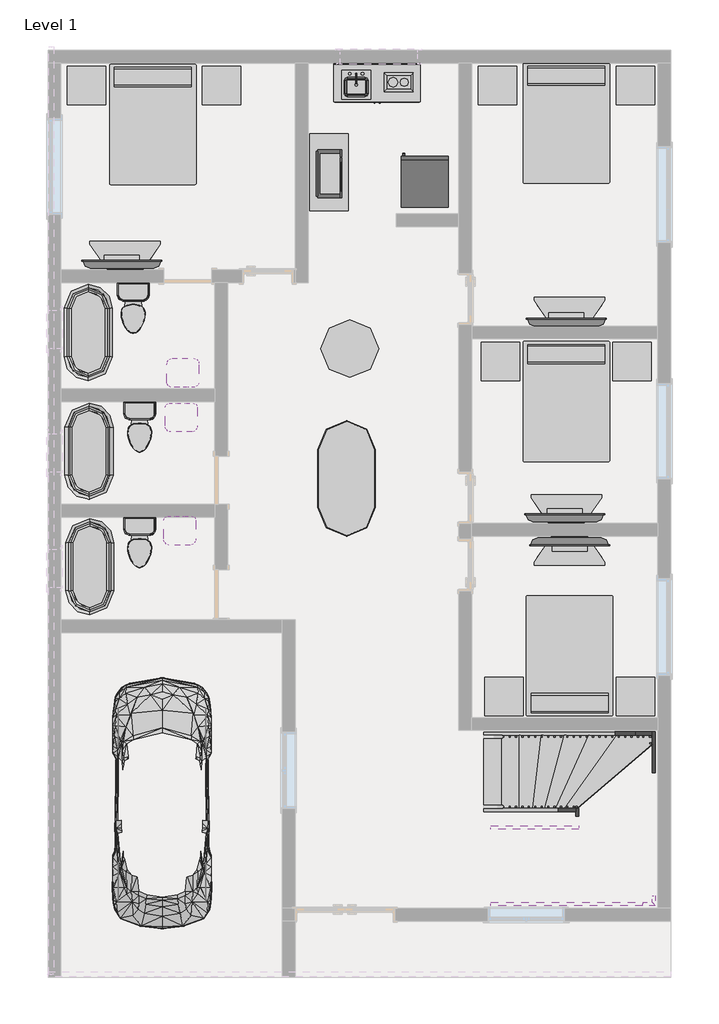
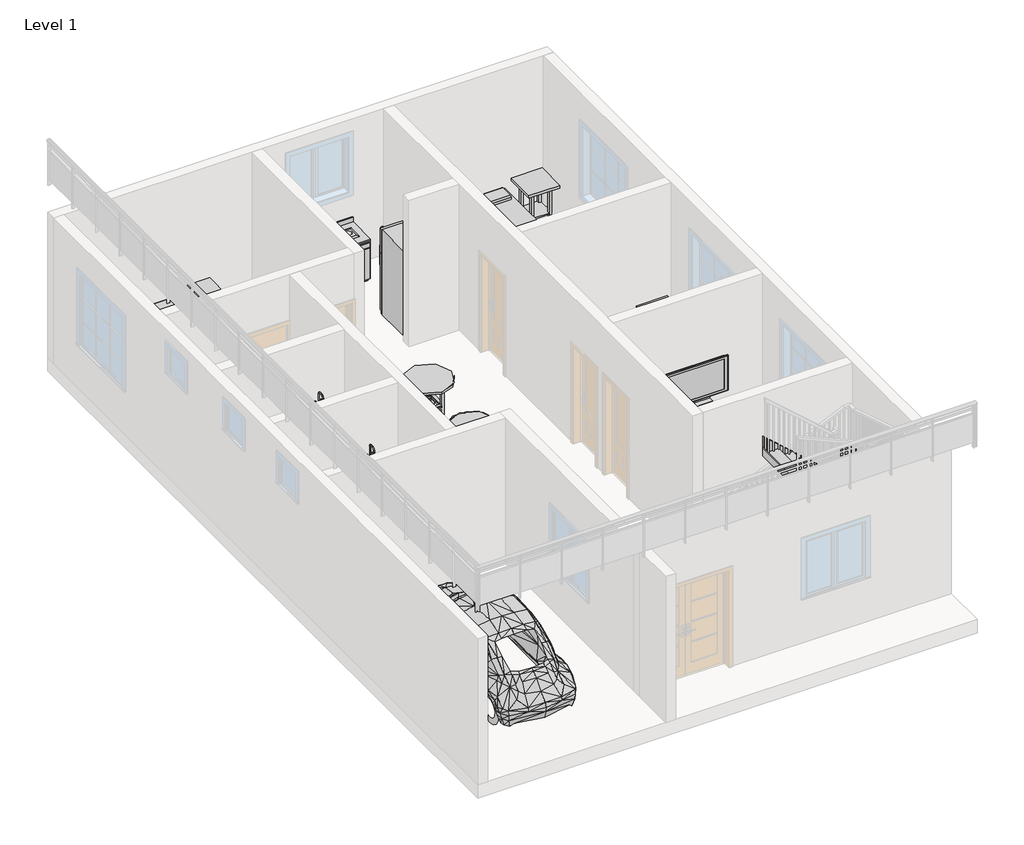
# One storey, part 4 of 4: 24 furniture elements, 10 flow terminals, 9 members, 5 proxies, 1 stair flight.
"""IFC4 building model written with IfcOpenShell, lengths in millimetres."""

from ifc_helpers import new_model, si_unit, frame, origin, place, context, project, spatial, polyline, outline, extrude, transform, mapped, element, save
from components import proxy_fe84b772, proxy_844211aa, proxy_8a8d5ab2, rpc_beetle_rpc_beetle_3ce7ba48, proxy_a13a33b2, flow_terminal_871c2e40, flow_terminal_62a433f7, toilet_domestic_3d_toilet_domestic_3d_f7549cf7, toilet_domestic_3d_toilet_domestic_3d_183bbd19, flow_terminal_b374fae2, furniture_0253826f, furniture_95afb093, furniture_fdf74506, tv_stand_tv_stand_6ce107e5, furniture_2c34a4f9, furniture_905aceb5, furniture_5bc9ed15, furniture_51091a24, stair_flight_e7964db3

model = new_model("IFC4")

# Units and contexts
model_context = context("Model", 3, world=origin())
ifc_project = project(units=[si_unit("LENGTHUNIT", "METRE", prefix="MILLI")], contexts=[model_context])

# Site, building, storey
site = spatial("IfcSite", under=ifc_project)
building = spatial("IfcBuilding", under=site)
storey = spatial("IfcBuildingStorey", under=building, Name="Level 1", Elevation=0.0)

# Proxies
placement = place(None, origin())
proxy_shape = proxy_fe84b772(model_context)
element("IfcBuildingElementProxy", 1, Name="Cook Top-2 Unit : 12\" x 18\"", ObjectType="Cook Top-2 Unit : 12\" x 18\"", at=placement, inside=storey, context=model_context, shape_type="MappedRepresentation", body=[
    mapped(proxy_shape, transform((-6638.6799646, 12850.7174997, 0.0), x_axis=(0.0, 1.0000000000000004, 0.0), y_axis=(-1.0000000000000004, 0.0, 0.0), z_axis=(0.0, 0.0, 1.0))),
])
proxy_2_shape = proxy_844211aa(model_context)
element("IfcBuildingElementProxy", 2, Name="Kitchenette - Small : 54\"", ObjectType="Kitchenette - Small : 54\"", at=placement, inside=storey, context=model_context, shape_type="MappedRepresentation", body=[
    mapped(proxy_2_shape, transform((-7030.5424651, 13231.7174997, 0.0), x_axis=(1.0000000000000004, 0.0, 0.0), y_axis=(0.0, 1.0000000000000004, 0.0), z_axis=(0.0, 0.0, 1.0))),
])
proxy_3_shape = proxy_8a8d5ab2(model_context)
element("IfcBuildingElementProxy", 3, Name="Microwave : 30\" x 16\" x 18\"", ObjectType="Microwave : 30\" x 16\" x 18\"", at=placement, inside=storey, context=model_context, shape_type="MappedRepresentation", body=[
    mapped(proxy_3_shape, transform((-8122.787078, 10978.8246223, 0.0), x_axis=(0.0, 1.000000000000001, 0.0), y_axis=(-1.000000000000001, 0.0, 0.0), z_axis=(0.0, 0.0, 1.0))),
])
rpc_beetle_rpc_beetle_shape = rpc_beetle_rpc_beetle_3ce7ba48(model_context)
element("IfcBuildingElementProxy", 4, Name="RPC Beetle : RPC Beetle", ObjectType="RPC Beetle : RPC Beetle", at=placement, inside=storey, context=model_context, shape_type="MappedRepresentation", body=[
    mapped(rpc_beetle_rpc_beetle_shape, transform((-10415.4047602, 277.7174997, 0.0), x_axis=(1.0, 0.0, 0.0), y_axis=(0.0, 1.0, 0.0), z_axis=(0.0, 0.0, 1.0))),
])
proxy_4_shape = proxy_a13a33b2(model_context)
element("IfcBuildingElementProxy", 5, Name="Refrigerator : 30\" x 32\" RH", ObjectType="Refrigerator : 30\" x 32\" RH", at=placement, inside=storey, context=model_context, shape_type="MappedRepresentation", body=[
    mapped(proxy_4_shape, transform((-6257.0375151, 11334.2664712, 0.0), x_axis=(-1.0000000000000002, 0.0, 0.0), y_axis=(0.0, -1.0000000000000002, 0.0), z_axis=(0.0, 0.0, 1.0))),
])

# Flow terminals
flow_terminal_shape = flow_terminal_871c2e40(model_context)
element("IfcFlowTerminal", 6, ObjectType="Sink Kitchen-Island : 18\" x 18\"", at=placement, inside=storey, context=model_context, shape_type="MappedRepresentation", body=[
    mapped(flow_terminal_shape, transform((-7357.6940008, 12886.4720986, 0.0), x_axis=(1.0000000000000004, 0.0, 0.0), y_axis=(0.0, 1.0000000000000004, 0.0), z_axis=(0.0, 0.0, 1.0))),
])
flow_terminal_2_shape = flow_terminal_62a433f7(model_context)
element("IfcFlowTerminal", 7, ObjectType="Sink Vanity-Square : 20\" x 18\"", at=placement, inside=storey, context=model_context, shape_type="MappedRepresentation", body=[
    mapped(flow_terminal_2_shape, transform((-10126.2940008, 7666.7720986, 914.4), x_axis=(1.0, 0.0, 0.0), y_axis=(0.0, 1.0, 0.0), z_axis=(0.0, 0.0, 1.0))),
])
element("IfcFlowTerminal", 8, ObjectType="Sink Vanity-Square : 20\" x 18\"", at=placement, inside=storey, context=model_context, shape_type="MappedRepresentation", body=[
    mapped(flow_terminal_2_shape, transform((-10069.5155196, 8281.0629008, 914.4), x_axis=(-1.0, 0.0, 0.0), y_axis=(0.0, -1.0, 0.0), z_axis=(0.0, 0.0, 1.0))),
])
element("IfcFlowTerminal", 9, ObjectType="Sink Vanity-Square : 20\" x 18\"", at=placement, inside=storey, context=model_context, shape_type="MappedRepresentation", body=[
    mapped(flow_terminal_2_shape, transform((-10151.6940008, 5876.0720986, 914.4), x_axis=(1.0, 0.0, 0.0), y_axis=(0.0, 1.0, 0.0), z_axis=(0.0, 0.0, 1.0))),
])
toilet_domestic_3d_toilet_domestic_3d_shape = toilet_domestic_3d_toilet_domestic_3d_f7549cf7(model_context)
toilet_domestic_3d_toilet_domestic_3d_2_shape = toilet_domestic_3d_toilet_domestic_3d_183bbd19(model_context)
element("IfcFlowTerminal", 10, ObjectType="Toilet-Domestic-3D : Toilet-Domestic-3D", at=placement, inside=storey, context=model_context, shape_type="MappedRepresentation", body=[
    mapped(toilet_domestic_3d_toilet_domestic_3d_shape, transform((-10770.6188676, 7377.6214723, 0.0), x_axis=(1.0, 0.0, 0.0), y_axis=(0.0, 1.0, 0.0), z_axis=(0.0, 0.0, 1.0))),
    mapped(toilet_domestic_3d_toilet_domestic_3d_2_shape, transform((-10770.6188676, 7377.6214723, 0.0), x_axis=(1.0, 0.0, 0.0), y_axis=(0.0, 1.0, 0.0), z_axis=(0.0, 0.0, 1.0))),
])
element("IfcFlowTerminal", 11, ObjectType="Toilet-Domestic-3D : Toilet-Domestic-3D", at=placement, inside=storey, context=model_context, shape_type="MappedRepresentation", body=[
    mapped(toilet_domestic_3d_toilet_domestic_3d_shape, transform((-10872.6047602, 9257.2214723, 0.0), x_axis=(1.0, 0.0, 0.0), y_axis=(0.0, 1.0, 0.0), z_axis=(0.0, 0.0, 1.0))),
    mapped(toilet_domestic_3d_toilet_domestic_3d_2_shape, transform((-10872.6047602, 9257.2214723, 0.0), x_axis=(1.0, 0.0, 0.0), y_axis=(0.0, 1.0, 0.0), z_axis=(0.0, 0.0, 1.0))),
])
element("IfcFlowTerminal", 12, ObjectType="Toilet-Domestic-3D : Toilet-Domestic-3D", at=placement, inside=storey, context=model_context, shape_type="MappedRepresentation", body=[
    mapped(toilet_domestic_3d_toilet_domestic_3d_shape, transform((-10770.6188676, 5548.8214723, 0.0), x_axis=(1.0, 0.0, 0.0), y_axis=(0.0, 1.0, 0.0), z_axis=(0.0, 0.0, 1.0))),
    mapped(toilet_domestic_3d_toilet_domestic_3d_2_shape, transform((-10770.6188676, 5548.8214723, 0.0), x_axis=(1.0, 0.0, 0.0), y_axis=(0.0, 1.0, 0.0), z_axis=(0.0, 0.0, 1.0))),
])
flow_terminal_3_shape = flow_terminal_b374fae2(model_context)
element("IfcFlowTerminal", 13, ObjectType="Tub-Free Standing-3D : 30\" x 60\"", at=placement, inside=storey, context=model_context, shape_type="MappedRepresentation", body=[
    mapped(flow_terminal_3_shape, transform((-11558.4047602, 5256.1174997, 0.0), x_axis=(1.0000000000000007, 0.0, 0.0), y_axis=(0.0, 1.0000000000000007, 0.0), z_axis=(0.0, 0.0, 1.0))),
])
element("IfcFlowTerminal", 14, ObjectType="Tub-Free Standing-3D : 30\" x 60\"", at=placement, inside=storey, context=model_context, shape_type="MappedRepresentation", body=[
    mapped(flow_terminal_3_shape, transform((-11571.7087329, 7084.313527, 0.0), x_axis=(1.0, 0.0, 0.0), y_axis=(0.0, 1.0, 0.0), z_axis=(0.0, 0.0, 1.0))),
])
element("IfcFlowTerminal", 15, ObjectType="Tub-Free Standing-3D : 30\" x 60\"", at=placement, inside=storey, context=model_context, shape_type="MappedRepresentation", body=[
    mapped(flow_terminal_3_shape, transform((-11583.8047602, 8964.5174997, 0.0), x_axis=(1.0, 0.0, 0.0), y_axis=(0.0, 1.0, 0.0), z_axis=(0.0, 0.0, 1.0))),
])

# Furniture
furniture_shape = furniture_0253826f(model_context)
element("IfcFurniture", 16, ObjectType="Bed-Standard.0001 : Double 54\" x 75\"", at=placement, inside=storey, context=model_context, shape_type="MappedRepresentation", body=[
    mapped(furniture_shape, transform((-3692.3162356, 3800.8224177, 0.0), x_axis=(-0.9999999999999998, 0.0, 0.0), y_axis=(0.0, -0.9999999999999998, 0.0), z_axis=(0.0, 0.0, 1.0))),
])
element("IfcFurniture", 17, ObjectType="Bed-Standard.0001 : Double 54\" x 75\"", at=placement, inside=storey, context=model_context, shape_type="MappedRepresentation", body=[
    mapped(furniture_shape, transform((-4286.0932848, 7917.9125816, 0.0), x_axis=(1.0000000000000002, 0.0, 0.0), y_axis=(0.0, 1.0000000000000002, 0.0), z_axis=(0.0, 0.0, 1.0))),
])
element("IfcFurniture", 18, ObjectType="Bed-Standard.0001 : Double 54\" x 75\"", at=placement, inside=storey, context=model_context, shape_type="MappedRepresentation", body=[
    mapped(furniture_shape, transform((-4286.0932848, 12324.8125816, 0.0), x_axis=(1.0, 0.0, 0.0), y_axis=(0.0, 1.0, 0.0), z_axis=(0.0, 0.0, 1.0))),
])
element("IfcFurniture", 19, ObjectType="Bed-Standard.0001 : Double 54\" x 75\"", at=placement, inside=storey, context=model_context, shape_type="MappedRepresentation", body=[
    mapped(furniture_shape, transform((-10832.9432848, 12305.7625816, 0.0), x_axis=(1.0, 0.0, 0.0), y_axis=(0.0, 1.0, 0.0), z_axis=(0.0, 0.0, 1.0))),
])
furniture_2_shape = furniture_95afb093(model_context)
element("IfcFurniture", 20, ObjectType="Counter Top w Sink Hole : 24\" Depth", at=placement, inside=storey, context=model_context, shape_type="MappedRepresentation", body=[
    mapped(furniture_2_shape, transform((-6497.1424651, 13231.7174997, 0.0), x_axis=(1.0000000000000004, 0.0, 0.0), y_axis=(0.0, 1.0000000000000004, 0.0), z_axis=(0.0, 0.0, 1.0))),
])
furniture_3_shape = furniture_fdf74506(model_context)
element("IfcFurniture", 21, ObjectType="TV - Flat Screen : 50\"", at=placement, inside=storey, context=model_context, shape_type="MappedRepresentation", body=[
    mapped(furniture_3_shape, transform((-11054.3492744, 10039.0561233, 914.4), x_axis=(-1.0000000000000002, 0.0, 0.0), y_axis=(0.0, -1.0000000000000002, 0.0), z_axis=(0.0, 0.0, 1.0))),
])
element("IfcFurniture", 22, ObjectType="TV - Flat Screen : 50\"", at=placement, inside=storey, context=model_context, shape_type="MappedRepresentation", body=[
    mapped(furniture_3_shape, transform((-4018.5492744, 9122.9549017, 914.4), x_axis=(-1.0, 0.0, 0.0), y_axis=(0.0, -1.0, 0.0), z_axis=(0.0, 0.0, 1.0))),
])
element("IfcFurniture", 23, ObjectType="TV - Flat Screen : 50\"", at=placement, inside=storey, context=model_context, shape_type="MappedRepresentation", body=[
    mapped(furniture_3_shape, transform((-4043.9492744, 6025.8561233, 914.4), x_axis=(-1.0, 0.0, 0.0), y_axis=(0.0, -1.0, 0.0), z_axis=(0.0, 0.0, 1.0))),
])
element("IfcFurniture", 24, ObjectType="TV - Flat Screen : 50\"", at=placement, inside=storey, context=model_context, shape_type="MappedRepresentation", body=[
    mapped(furniture_3_shape, transform((-3959.8602461, 5654.778876, 914.4), x_axis=(1.0, 0.0, 0.0), y_axis=(0.0, 1.0, 0.0), z_axis=(0.0, 0.0, 1.0))),
])
tv_stand_tv_stand_shape = tv_stand_tv_stand_6ce107e5(model_context)
element("IfcFurniture", 25, ObjectType="TV Stand : TV Stand", at=placement, inside=storey, context=model_context, shape_type="MappedRepresentation", body=[
    mapped(tv_stand_tv_stand_shape, transform((-10874.4167581, 9955.1174997, 0.0), x_axis=(-1.0000000000000004, 0.0, 0.0), y_axis=(0.0, -1.0000000000000004, 0.0), z_axis=(0.0, 0.0, 1.0))),
])
element("IfcFurniture", 26, ObjectType="TV Stand : TV Stand", at=placement, inside=storey, context=model_context, shape_type="MappedRepresentation", body=[
    mapped(tv_stand_tv_stand_shape, transform((-3838.6167581, 9066.1174997, 0.0), x_axis=(-1.0, 0.0, 0.0), y_axis=(0.0, -1.0, 0.0), z_axis=(0.0, 0.0, 1.0))),
])
element("IfcFurniture", 27, ObjectType="TV Stand : TV Stand", at=placement, inside=storey, context=model_context, shape_type="MappedRepresentation", body=[
    mapped(tv_stand_tv_stand_shape, transform((-3889.4167581, 5941.9174997, 0.0), x_axis=(-1.0, 0.0, 0.0), y_axis=(0.0, -1.0, 0.0), z_axis=(0.0, 0.0, 1.0))),
])
element("IfcFurniture", 28, ObjectType="TV Stand : TV Stand", at=placement, inside=storey, context=model_context, shape_type="MappedRepresentation", body=[
    mapped(tv_stand_tv_stand_shape, transform((-4088.9927623, 5738.7174997, 0.0), x_axis=(1.0000000000000002, 0.0, 0.0), y_axis=(0.0, 1.0000000000000002, 0.0), z_axis=(0.0, 0.0, 1.0))),
])
furniture_4_shape = furniture_2c34a4f9(model_context)
element("IfcFurniture", 29, ObjectType="Table-Dining Oval : 36\" x 72\"", at=placement, inside=storey, context=model_context, shape_type="MappedRepresentation", body=[
    mapped(furniture_4_shape, transform((-7852.5031209, 7054.9371718, 0.0), x_axis=(0.0, 1.0000000000000002, 0.0), y_axis=(-1.0000000000000002, 0.0, 0.0), z_axis=(0.0, 0.0, 1.0))),
])
furniture_5_shape = furniture_905aceb5(model_context)
element("IfcFurniture", 30, ObjectType="Table-Dining Round w Chairs : 36\" Diameter", at=placement, inside=storey, context=model_context, shape_type="MappedRepresentation", body=[
    mapped(furniture_5_shape, transform((-7547.2867274, 8895.3961882, 0.0), x_axis=(1.0, 0.0, 0.0), y_axis=(0.0, 1.0, 0.0), z_axis=(0.0, 0.0, 1.0))),
])
furniture_6_shape = furniture_5bc9ed15(model_context)
element("IfcFurniture", 31, ObjectType="Table-Night Stand : 24\" x 24\" x 30\"", at=placement, inside=storey, context=model_context, shape_type="MappedRepresentation", body=[
    mapped(furniture_6_shape, transform((-11917.7383905, 12571.3174997, 0.0), x_axis=(1.0, 0.0, 0.0), y_axis=(0.0, 1.0, 0.0), z_axis=(0.0, 0.0, 1.0))),
])
element("IfcFurniture", 32, ObjectType="Table-Night Stand : 24\" x 24\" x 30\"", at=placement, inside=storey, context=model_context, shape_type="MappedRepresentation", body=[
    mapped(furniture_6_shape, transform((-9784.1383905, 12571.3174997, 0.0), x_axis=(1.0, 0.0, 0.0), y_axis=(0.0, 1.0, 0.0), z_axis=(0.0, 0.0, 1.0))),
])
element("IfcFurniture", 33, ObjectType="Table-Night Stand : 24\" x 24\" x 30\"", at=placement, inside=storey, context=model_context, shape_type="MappedRepresentation", body=[
    mapped(furniture_6_shape, transform((-5415.3383905, 12571.3174997, 0.0), x_axis=(1.0, 0.0, 0.0), y_axis=(0.0, 1.0, 0.0), z_axis=(0.0, 0.0, 1.0))),
])
element("IfcFurniture", 34, ObjectType="Table-Night Stand : 24\" x 24\" x 30\"", at=placement, inside=storey, context=model_context, shape_type="MappedRepresentation", body=[
    mapped(furniture_6_shape, transform((-3230.9383905, 12571.3174997, 0.0), x_axis=(1.0, 0.0, 0.0), y_axis=(0.0, 1.0, 0.0), z_axis=(0.0, 0.0, 1.0))),
])
element("IfcFurniture", 35, ObjectType="Table-Night Stand : 24\" x 24\" x 30\"", at=placement, inside=storey, context=model_context, shape_type="MappedRepresentation", body=[
    mapped(furniture_6_shape, transform((-5364.5383905, 8202.5174997, 0.0), x_axis=(1.0, 0.0, 0.0), y_axis=(0.0, 1.0, 0.0), z_axis=(0.0, 0.0, 1.0))),
])
element("IfcFurniture", 36, ObjectType="Table-Night Stand : 24\" x 24\" x 30\"", at=placement, inside=storey, context=model_context, shape_type="MappedRepresentation", body=[
    mapped(furniture_6_shape, transform((-3281.7383905, 8202.5174997, 0.0), x_axis=(1.0, 0.0, 0.0), y_axis=(0.0, 1.0, 0.0), z_axis=(0.0, 0.0, 1.0))),
])
element("IfcFurniture", 37, ObjectType="Table-Night Stand : 24\" x 24\" x 30\"", at=placement, inside=storey, context=model_context, shape_type="MappedRepresentation", body=[
    mapped(furniture_6_shape, transform((-3230.9383905, 2893.9174997, 0.0), x_axis=(1.0, 0.0, 0.0), y_axis=(0.0, 1.0, 0.0), z_axis=(0.0, 0.0, 1.0))),
])
element("IfcFurniture", 38, ObjectType="Table-Night Stand : 24\" x 24\" x 30\"", at=placement, inside=storey, context=model_context, shape_type="MappedRepresentation", body=[
    mapped(furniture_6_shape, transform((-5313.7383905, 2893.9174997, 0.0), x_axis=(1.0, 0.0, 0.0), y_axis=(0.0, 1.0, 0.0), z_axis=(0.0, 0.0, 1.0))),
])
furniture_7_shape = furniture_51091a24(model_context)
element("IfcFurniture", 39, ObjectType="Table-Rectangular : 72\" x 30\"", at=placement, inside=storey, context=model_context, shape_type="MappedRepresentation", body=[
    mapped(furniture_7_shape, transform((-7773.8047602, 11504.5174997, 0.0), x_axis=(0.0, 1.0, 0.0), y_axis=(-1.0, 0.0, 0.0), z_axis=(0.0, 0.0, 1.0))),
])

# Members
element("IfcMember", 40, ObjectType="Stringer - 2\" Width", at=placement, inside=storey, context=model_context, shape_type="SweptSolid", body=[
    extrude(outline(polyline([(240.2084845, -5318.5510787), (0.0, -5318.5510787), (0.0, -5112.044989), (1015.0127538, -2923.6509652), (1351.0021226, -2923.6509652), (240.2084845, -5318.5510787)])), frame((0.0, 2589.1174997, 0.0), z_axis=(0.0, 1.0, 0.0), x_axis=(0.0, 0.0, 1.0)), (0.0, 0.0, 1.0), 50.8),
])
element("IfcMember", 41, ObjectType="Stringer - 2\" Width", at=placement, inside=storey, context=model_context, shape_type="SweptSolid", body=[
    extrude(outline(polyline([(-2923.6509652, 2589.1174997), (-2923.6509652, 2639.9174997), (-2657.7693695, 2639.9174997), (-2657.7693695, 2589.1174997), (-2923.6509652, 2589.1174997)])), frame((0.0, 0.0, 1015.0127538), z_axis=(0.0, 0.0, 1.0), x_axis=(1.0, 0.0, 0.0)), (0.0, 0.0, 1.0), 335.9893688),
])
element("IfcMember", 42, ObjectType="Stringer - 2\" Width", at=placement, inside=storey, context=model_context, shape_type="SweptSolid", body=[
    extrude(outline(polyline([(2639.9174997, 1335.0931561), (2639.9174997, 1046.2021226), (2489.5246107, 1046.2021226), (44.8121446, 1811.8093816), (44.8121446, 2147.7987504), (2639.9174997, 1335.0931561)])), frame((-2657.7693695, 0.0, 0.0), z_axis=(1.0, 0.0, 0.0), x_axis=(0.0, 1.0, 0.0)), (0.0, 0.0, 1.0), 50.8),
])
element("IfcMember", 43, ObjectType="Stringer - 2\" Width", at=placement, inside=storey, context=model_context, shape_type="SweptSolid", body=[
    extrude(outline(polyline([(-2657.7693695, 44.8121446), (-2606.9693695, 44.8121446), (-2606.9693695, -107.8172843), (-2657.7693695, -57.0172843), (-2657.7693695, 44.8121446)])), frame((0.0, 0.0, 1820.0491797), z_axis=(0.0, 0.0, 1.0), x_axis=(1.0, 0.0, 0.0)), (0.0, 0.0, 1.0), 319.3970378),
])
element("IfcMember", 44, ObjectType="Stringer - 2\" Width", at=placement, inside=storey, context=model_context, shape_type="SweptSolid", body=[
    extrude(outline(polyline([(-2657.7693695, -57.0172843), (-2606.9693695, -107.8172843), (-2802.7898914, -107.8172843), (-2802.7898914, -57.0172843), (-2657.7693695, -57.0172843)])), frame((0.0, 0.0, 1820.0491797), z_axis=(0.0, 0.0, 1.0), x_axis=(1.0, 0.0, 0.0)), (0.0, 0.0, 1.0), 319.3970378),
])
element("IfcMember", 45, ObjectType="Stringer - 2\" Width", at=placement, inside=storey, context=model_context, shape_type="SweptSolid", body=[
    extrude(outline(polyline([(1820.0491797, -2802.7898914), (2139.4462175, -2802.7898914), (3193.0858569, -5209.7542153), (2873.6888191, -5209.7542153), (1820.0491797, -2802.7898914)])), frame((0.0, -107.8172843, 0.0), z_axis=(0.0, 1.0, 0.0), x_axis=(0.0, 0.0, 1.0)), (0.0, 0.0, 1.0), 50.8),
])
element("IfcMember", 46, ObjectType="Stringer - 2\" Width", at=placement, inside=storey, context=model_context, shape_type="SweptSolid", body=[
    extrude(outline(polyline([(166.5746126, -5318.5510787), (0.0, -5318.5510787), (0.0, -5046.2345701), (1034.8273187, -3866.5367614), (1440.2771419, -3866.5367614), (166.5746126, -5318.5510787)])), frame((0.0, 1380.3501077, 0.0), z_axis=(0.0, 1.0, 0.0), x_axis=(0.0, 0.0, 1.0)), (0.0, 0.0, 1.0), 50.8),
])
element("IfcMember", 47, ObjectType="Stringer - 2\" Width", at=placement, inside=storey, context=model_context, shape_type="SweptSolid", body=[
    extrude(outline(polyline([(1431.1501077, 1636.067451), (1431.1501077, 1079.3889237), (1365.5854639, 1079.3889237), (1151.7501077, 1513.5060424), (1151.7501077, 2137.2957264), (1184.2574555, 2137.2957264), (1431.1501077, 1636.067451)])), frame((-3866.5367614, 0.0, 0.0), z_axis=(1.0, 0.0, 0.0), x_axis=(0.0, 1.0, 0.0)), (0.0, 0.0, 1.0), 50.8),
])
element("IfcMember", 48, ObjectType="Stringer - 2\" Width", at=placement, inside=storey, context=model_context, shape_type="SweptSolid", body=[
    extrude(outline(polyline([(1730.6293364, -3815.7367614), (2137.2957264, -3815.7367614), (3368.5447543, -5209.7542153), (2961.8783644, -5209.7542153), (1730.6293364, -3815.7367614)])), frame((0.0, 1100.9501077, 0.0), z_axis=(0.0, 1.0, 0.0), x_axis=(0.0, 0.0, 1.0)), (0.0, 0.0, 1.0), 50.8),
])

# Stair flight
stair_flight_shape = stair_flight_e7964db3(model_context)
element("IfcStairFlight", 49, ObjectType="2\" Tread 1\" Nosing 1/4\" Riser", at=placement, inside=storey, context=model_context, shape_type="MappedRepresentation", body=[
    mapped(stair_flight_shape, transform((0.0, 0.0, 0.0), x_axis=(1.0, 0.0, 0.0), y_axis=(0.0, 1.0, 0.0), z_axis=(0.0, 0.0, 1.0))),
])

save(model, "model.ifc")

# Revit data of these elements
# Type "Cook Top-2 Unit : 12\" x 18\""
#   Assembly Code = "E1090400"
#   Counter Height = 3' - 0"
#   Depth = 1' - 6"
#   Width = 1' - 0"
#   Burner Material = Steel, Chrome Plated
#   Cooktop Material = Steel, Polished
#   Default Elevation = 0
# Type "Kitchenette - Small : 54\""
#   Assembly Code = "E1090400"
#   Width = 4' - 6"
#   Height = 2' - 10 1/2"
#   Depth = 2' - 0"
#   Toe Depth = 0' - 3"
#   Toe Height = 0' - 3 1/2"
#   Cabinet Material = Cabinets
#   Door/Drawer Material = Cabinets
#   Handle Material = Cabinets - Handles
#   Default Elevation = 0
# Type "Microwave : 30\" x 16\" x 18\""
#   Assembly Code = "E1090400"
#   Depth = 1' - 4"
#   Height = 1' - 6"
#   Width = 2' - 6"
#   Microwave Material = Laminate, Ivory, Matte
#   Default Elevation = 0
# Type "RPC Beetle : RPC Beetle"
#   built-in parameter 1005195 = "RPC-16-0U6E-L4EG-ENH1-J3KF-SVEL-0TX4-C0"
#   Height = 0
# Type "Refrigerator : 30\" x 32\" RH"
#   Label = "REF."
#   Assembly Code = "E1090400"
#   Depth = 2' - 7 3/4"
#   Handle = 2' - 3"
#   Height = 5' - 10"
#   Rear Clearance = 0' - 2"
#   Top Door Height = 1' - 8"
#   Width = 2' - 5 3/8"
#   Material = Steel, Paint Finish, Ivory, Glossy
#   Default Elevation = 0
# Type "Sink Kitchen-Island : 18\" x 18\""
#   Assembly Code = "D2010410"
#   Counter Height = 3' - 0"
#   Depth = 1' - 6"
#   Width = 1' - 6"
#   Faucet Material = Steel, Polished
#   Sink Material = Steel, Polished
#   Default Elevation = 0
# Type "Sink Vanity-Square : 20\" x 18\""
#   Assembly Code = "D2010400"
#   Counter Height = 2' - 7"
#   Depth = 1' - 6"
#   Width = 1' - 8"
#   Basin Material = Porcelain, Linen
#   Faucet Material = Steel, Polished
#   Default Elevation = 0
# Type "Toilet-Domestic-3D : Toilet-Domestic-3D"
#   Assembly Code = "D2010110"
#   Toilet - Bowl/Basin Material = Porcelain, Linen
#   Toilet - Seat Material = Laminate, Linen, Matte
#   Default Elevation = 0
# Type "Tub-Free Standing-3D : 30\" x 60\""
#   Assembly Code = "D2010110"
#   Height = 1' - 6"
#   Length = 5' - 0"
#   Width = 2' - 6"
#   Tub Material = Porcelain, Ivory
#   Default Elevation = 0
# Type "Bed-Standard.0001 : Double 54\" x 75\""
#   Assembly Code = "E2020200"
#   Length = 6' - 3"
#   Width = 4' - 6"
#   Leg Material = Steel, Chrome Plated
#   Mattress Material = Linen, White
#   Default Elevation = 0
# Type "Counter Top w Sink Hole : 24\" Depth"
#   Assembly Code = "C1030400"
#   Counter Thickness = 0' - 1 1/2"
#   Depth [instance default] = 2' - 1"
#   Height = 3' - 0"
#   Length [instance default] = 8' - 0"
#   Sink Location [instance default] = 2' - 0"
#   Sink Location To Wall [instance default] = 0' - 6"
#   Sink Opening Depth [instance default] = 1' - 3"
#   Sink Opening Width [instance default] = 2' - 3"
#   Counter Top Material = none
#   Default Elevation = 0
# Type "TV - Flat Screen : 50\""
#   SinAng = 0' - 0.0193"
#   L = 3' - 7.57782"
#   H = 2' - 0.51477"
#   Thickness = 0' - 4.33071"
#   Diagonal = 4' - 2"
#   CosAng = 0' - 0.03431"
#   Stand [instance default] = yes
#   Default Elevation = 0
# Type "TV Stand : TV Stand"
#   Depth = 1' - 6"
#   Width = 3' - 8"
#   Height = 1' - 7 1/2"
#   Finish = Melamine - Gray
#   Default Elevation = 0
# Type "Table-Dining Oval : 36\" x 72\""
#   Assembly Code = "E2020200"
#   Length = 6' - 0"
#   Width = 3' - 0"
#   Base Material = Steel, Chrome Plated
#   Top Material = Glass - Clear, Grey
#   Default Elevation = 0
#   Description = (empty or 0)
# Type "Table-Dining Round w Chairs : 36\" Diameter"
#   Assembly Code = "E2020200"
#   Radius = 1' - 6"
#   Diameter = 3' - 0"
#   Height = 2' - 6"
#   Chairs = 4
#   Base Material = Pine
#   Top Material = Laminate, Linen, Matte
#   Default Elevation = 0
# Type "Table-Night Stand : 24\" x 24\" x 30\""
#   Assembly Code = "E2020200"
#   Depth = 2' - 0"
#   Height = 2' - 6"
#   Width = 2' - 0"
#   Base Material = Birch
#   Top Material = Laminate, Ivory, Matte
#   Default Elevation = 0
# Type "Table-Rectangular : 72\" x 30\""
#   Assembly Code = "E2020200"
#   Height = 2' - 6"
#   Length = 4' - 0"
#   Width = 2' - 0"
#   Base Material = Birch
#   Top Material = Birch
#   Default Elevation = 0
# Element 1 (IfcBuildingElementProxy, "Cook Top-2 Unit : 12\" x 18\"")
#   Phase Created = New Construction
#   Materials on its faces: "Steel, Chrome Plated", "Steel, Polished"
# Element 2 (IfcBuildingElementProxy, "Kitchenette - Small : 54\"")
#   Phase Created = New Construction
#   Materials on its faces: "Cabinets", "Cabinets - Handles"
# Element 3 (IfcBuildingElementProxy, "Microwave : 30\" x 16\" x 18\"")
#   Phase Created = New Construction
#   Materials on its faces: "Laminate, Ivory, Matte", "Glass"
# Element 4 (IfcBuildingElementProxy, "RPC Beetle : RPC Beetle")
#   Phase Created = New Construction
# Element 5 (IfcBuildingElementProxy, "Refrigerator : 30\" x 32\" RH")
#   Phase Created = New Construction
#   Materials on its faces: "Steel, Paint Finish, Ivory, Glossy", "Steel, Chrome Plated"
# Element 6 (IfcFlowTerminal, "Sink Kitchen-Island : 18\" x 18\"")
#   Mark = "15"
#   Phase Created = New Construction
#   Materials on its faces: "Steel, Polished"
# Element 7 (IfcFlowTerminal, "Sink Vanity-Square : 20\" x 18\"")
#   Mark = "12"
#   Phase Created = New Construction
#   Materials on its faces: "Porcelain, Linen", "Steel, Polished"
# Element 8 (IfcFlowTerminal, "Sink Vanity-Square : 20\" x 18\"")
#   Mark = "13"
#   Phase Created = New Construction
#   Materials on its faces: "Porcelain, Linen", "Steel, Polished"
# Element 9 (IfcFlowTerminal, "Sink Vanity-Square : 20\" x 18\"")
#   Mark = "14"
#   Phase Created = New Construction
#   Materials on its faces: "Porcelain, Linen", "Steel, Polished"
# Element 10 (IfcFlowTerminal, "Toilet-Domestic-3D : Toilet-Domestic-3D")
#   Mark = "7"
#   Phase Created = New Construction
#   Materials on its faces: "Porcelain, Linen", "Laminate, Linen, Matte"
# Element 11 (IfcFlowTerminal, "Toilet-Domestic-3D : Toilet-Domestic-3D")
#   Mark = "8"
#   Phase Created = New Construction
#   Materials on its faces: "Porcelain, Linen", "Laminate, Linen, Matte"
# Element 12 (IfcFlowTerminal, "Toilet-Domestic-3D : Toilet-Domestic-3D")
#   Mark = "9"
#   Phase Created = New Construction
#   Materials on its faces: "Porcelain, Linen", "Laminate, Linen, Matte"
# Element 13 (IfcFlowTerminal, "Tub-Free Standing-3D : 30\" x 60\"")
#   Mark = "4"
#   Phase Created = New Construction
#   Materials on its faces: "Porcelain, Ivory"
# Element 14 (IfcFlowTerminal, "Tub-Free Standing-3D : 30\" x 60\"")
#   Mark = "5"
#   Phase Created = New Construction
#   Materials on its faces: "Porcelain, Ivory"
# Element 15 (IfcFlowTerminal, "Tub-Free Standing-3D : 30\" x 60\"")
#   Mark = "6"
#   Phase Created = New Construction
#   Materials on its faces: "Porcelain, Ivory"
# Elements 16, 17, 18, 19 (IfcFurniture, "Bed-Standard.0001 : Double 54\" x 75\"")
#   Phase Created = New Construction
#   Materials on its faces: "Linen, White", "Steel, Chrome Plated"
# Element 20 (IfcFurniture, "Counter Top w Sink Hole : 24\" Depth")
#   Sink Opening Depth = 1' - 3"
#   Sink Location To Wall = 0' - 6"
#   Length = 4' - 6"
#   Sink Location = 1' - 2"
#   Sink Opening Width = 1' - 4"
#   Depth = 2' - 0"
#   Phase Created = New Construction
#   Materials on its faces: "Counter Top"
# Elements 21, 22, 23, 24 (IfcFurniture, "TV - Flat Screen : 50\"")
#   Stand = yes
#   Phase Created = New Construction
#   Materials on its faces: "TV - Black", "TV - Glass", "TV - Screen"
# Elements 25, 26, 27, 28 (IfcFurniture, "TV Stand : TV Stand")
#   Phase Created = New Construction
#   Materials on its faces: "Melamine - Gray", "Glass - Shelves"
# Element 29 (IfcFurniture, "Table-Dining Oval : 36\" x 72\"")
#   Phase Created = New Construction
#   Materials on its faces: "Steel, Chrome Plated", "Glass - Clear, Grey"
# Element 30 (IfcFurniture, "Table-Dining Round w Chairs : 36\" Diameter")
#   Phase Created = New Construction
#   Materials on its faces: "Pine", "Laminate, Linen, Matte"
# Elements 31, 32, 33, 34, 35, 36, 37, 38 (IfcFurniture, "Table-Night Stand : 24\" x 24\" x 30\"")
#   Phase Created = New Construction
#   Materials on its faces: "Birch", "Laminate, Ivory, Matte"
# Element 39 (IfcFurniture, "Table-Rectangular : 72\" x 30\"")
#   Phase Created = New Construction
#   Materials on its faces: "Birch"
# Elements 40, 41, 42, 43, 44, 45, 46, 47, 48 (IfcMember, "Stringer - 2\" Width")
#   Phase Created = New Construction
# Element 49 (IfcStairFlight, "2\" Tread 1\" Nosing 1/4\" Riser")
#   Phase Created = New Construction
# Materials
#   "Steel, Chrome Plated": class "Metal", colour RGB 17 17 17, transparency 0, Description = "Chromiuim plated steel", Cost = 0
#   "Steel, Polished": class "Metal", colour RGB 57 57 57, transparency 0, Description = "Polished steel", Cost = 0
#   "Cabinets": colour RGB 249 249 249, transparency 0
#   "Cabinets - Handles": class "Metal", colour RGB 57 57 57, transparency 0
#   "Laminate, Ivory, Matte": class "Plastic", colour RGB 247 247 239, transparency 0, Description = "Plastic Laminate - Ivory, Matte", Cost = 0
#   "Steel, Paint Finish, Ivory, Glossy": class "Metal", colour RGB 247 247 239, transparency 0, Description = "Steel, paint finish, ivory, glossy", Cost = 0
#   "Porcelain, Linen": class "Ceramic", colour RGB 249 239 230, transparency 0, Description = "Porcelain, linen", Cost = 0
#   "Laminate, Linen, Matte": class "Plastic", colour RGB 249 239 230, transparency 0, Description = "Plastic Laminate - Linen, Matte", Cost = 0
#   "Porcelain, Ivory": class "Ceramic", colour RGB 247 247 239, transparency 0, Description = "Porcelain, ivory", Cost = 0
#   "Linen, White": class "Textile", colour RGB 247 247 239, transparency 0, Description = "Linen, white", Cost = 0
#   "Melamine - Gray": class "Wood", colour RGB 49 49 49, transparency 0
#   "Glass - Clear, Grey": class "Glass", colour RGB 252 255 255, transparency 0.64
#   "Pine": class "Wood", colour RGB 223 192 134, transparency 0, Description = "Pinus Echinata", Cost = 0
#   "Birch": class "Wood", colour RGB 224 178 126, transparency 0, Description = "Betula Alleghaniensis", Cost = 0
#   "Glass": class "Glass", colour RGB 0 128 192, transparency 0.75, Description = "Soda Lime Glass", Cost = 0
#   "Counter Top": class "Wood", colour RGB 226 177 128, transparency 0
#   "TV - Black": colour RGB 49 49 49, transparency 0
#   "TV - Glass": colour RGB 157 157 157, transparency 0.9
#   "TV - Screen": colour RGB 0 0 0, transparency 0
#   "Glass - Shelves": class "Glass", colour RGB 167 167 167, transparency 0.9
